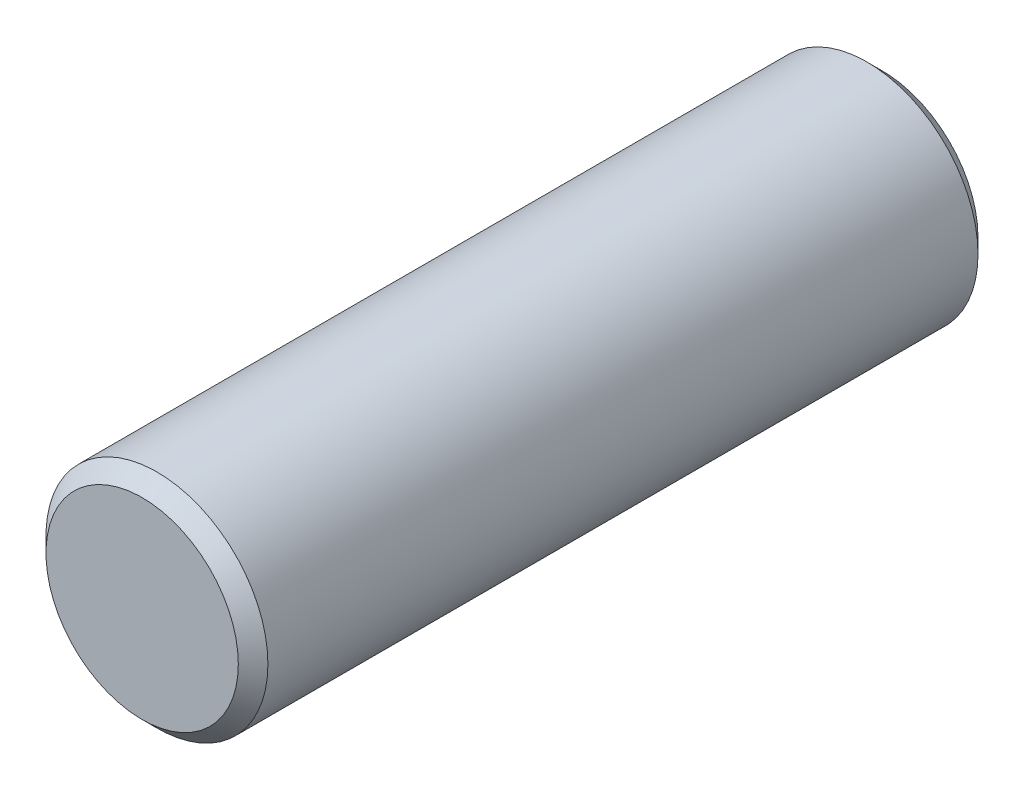
ISO-10303-21;
HEADER;
FILE_DESCRIPTION(('STEP AP214'),'2;1');
FILE_NAME('part.step','',(''),(''),'','','');
FILE_SCHEMA(('AUTOMOTIVE_DESIGN { 1 0 10303 214 1 1 1 1 }'));
ENDSEC;
DATA;
#1=APPLICATION_CONTEXT('core data for automotive mechanical design processes');
#2=APPLICATION_PROTOCOL_DEFINITION('international standard','automotive_design',2000,#1);
#3=PRODUCT_CONTEXT('',#1,'mechanical');
#4=PRODUCT('Part','Part','',(#3));
#5=PRODUCT_RELATED_PRODUCT_CATEGORY('part','',(#4));
#6=PRODUCT_DEFINITION_FORMATION('','',#4);
#7=PRODUCT_DEFINITION_CONTEXT('part definition',#1,'design');
#8=PRODUCT_DEFINITION('design','',#6,#7);
#9=PRODUCT_DEFINITION_SHAPE('','',#8);
#10=(LENGTH_UNIT() NAMED_UNIT(*) SI_UNIT(.MILLI.,.METRE.));
#11=(NAMED_UNIT(*) PLANE_ANGLE_UNIT() SI_UNIT($,.RADIAN.));
#12=(NAMED_UNIT(*) SI_UNIT($,.STERADIAN.) SOLID_ANGLE_UNIT());
#13=UNCERTAINTY_MEASURE_WITH_UNIT(LENGTH_MEASURE(1.E-05),#10,'distance_accuracy_value','');
#14=(GEOMETRIC_REPRESENTATION_CONTEXT(3) GLOBAL_UNCERTAINTY_ASSIGNED_CONTEXT((#13)) GLOBAL_UNIT_ASSIGNED_CONTEXT((#10,
#11,#12)) REPRESENTATION_CONTEXT('',''));
#15=CARTESIAN_POINT('',(0.,0.,0.));
#16=DIRECTION('',(0.,0.,1.));
#17=DIRECTION('',(1.,0.,0.));
#18=AXIS2_PLACEMENT_3D('',#15,#16,#17);
#19=CARTESIAN_POINT('',(0.,0.,5.));
#20=DIRECTION('',(0.,0.,-1.));
#21=DIRECTION('',(-1.,0.,0.));
#22=AXIS2_PLACEMENT_3D('',#19,#20,#21);
#23=CYLINDRICAL_SURFACE('',#22,1.5);
#24=CARTESIAN_POINT('',(0.,0.,-4.8));
#25=DIRECTION('',(0.,0.,1.));
#26=DIRECTION('',(1.,0.,0.));
#27=AXIS2_PLACEMENT_3D('',#24,#25,#26);
#28=CIRCLE('',#27,1.5);
#29=CARTESIAN_POINT('',(1.5,0.,-4.8));
#30=VERTEX_POINT('',#29);
#31=EDGE_CURVE('E51',#30,#30,#28,.T.);
#32=ORIENTED_EDGE('',*,*,#31,.T.);
#33=EDGE_LOOP('',(#32));
#34=FACE_BOUND('',#33,.T.);
#35=CARTESIAN_POINT('',(0.,0.,4.8));
#36=DIRECTION('',(0.,0.,1.));
#37=DIRECTION('',(1.,0.,0.));
#38=AXIS2_PLACEMENT_3D('',#35,#36,#37);
#39=CIRCLE('',#38,1.5);
#40=CARTESIAN_POINT('',(1.5,0.,4.8));
#41=VERTEX_POINT('',#40);
#42=EDGE_CURVE('E54',#41,#41,#39,.F.);
#43=ORIENTED_EDGE('',*,*,#42,.T.);
#44=EDGE_LOOP('',(#43));
#45=FACE_BOUND('',#44,.T.);
#46=ADVANCED_FACE('F39',(#34,#45),#23,.T.);
#47=CARTESIAN_POINT('',(0.,0.,5.));
#48=DIRECTION('',(0.,0.,1.));
#49=DIRECTION('',(1.,0.,0.));
#50=AXIS2_PLACEMENT_3D('',#47,#48,#49);
#51=PLANE('',#50);
#52=CARTESIAN_POINT('',(0.,0.,5.));
#53=DIRECTION('',(0.,0.,1.));
#54=DIRECTION('',(1.,0.,0.));
#55=AXIS2_PLACEMENT_3D('',#52,#53,#54);
#56=CIRCLE('',#55,1.3);
#57=CARTESIAN_POINT('',(1.3,0.,5.));
#58=VERTEX_POINT('',#57);
#59=EDGE_CURVE('E10',#58,#58,#56,.T.);
#60=ORIENTED_EDGE('',*,*,#59,.T.);
#61=EDGE_LOOP('',(#60));
#62=FACE_BOUND('',#61,.T.);
#63=ADVANCED_FACE('F72',(#62),#51,.T.);
#64=CARTESIAN_POINT('',(0.,0.,-5.));
#65=DIRECTION('',(0.,0.,1.));
#66=DIRECTION('',(1.,0.,0.));
#67=AXIS2_PLACEMENT_3D('',#64,#65,#66);
#68=PLANE('',#67);
#69=CARTESIAN_POINT('',(0.,0.,-5.));
#70=DIRECTION('',(0.,0.,1.));
#71=DIRECTION('',(1.,0.,0.));
#72=AXIS2_PLACEMENT_3D('',#69,#70,#71);
#73=CIRCLE('',#72,1.3);
#74=CARTESIAN_POINT('',(1.3,0.,-5.));
#75=VERTEX_POINT('',#74);
#76=EDGE_CURVE('E50',#75,#75,#73,.F.);
#77=ORIENTED_EDGE('',*,*,#76,.T.);
#78=EDGE_LOOP('',(#77));
#79=FACE_BOUND('',#78,.T.);
#80=ADVANCED_FACE('F70',(#79),#68,.F.);
#81=CARTESIAN_POINT('',(0.,0.,-4.8));
#82=DIRECTION('',(0.,0.,1.));
#83=DIRECTION('',(1.,0.,0.));
#84=AXIS2_PLACEMENT_3D('',#81,#82,#83);
#85=CONICAL_SURFACE('',#84,1.5,0.785398163397452);
#86=ORIENTED_EDGE('',*,*,#76,.F.);
#87=EDGE_LOOP('',(#86));
#88=FACE_BOUND('',#87,.T.);
#89=ORIENTED_EDGE('',*,*,#31,.F.);
#90=EDGE_LOOP('',(#89));
#91=FACE_BOUND('',#90,.T.);
#92=ADVANCED_FACE('F63',(#88,#91),#85,.T.);
#93=CARTESIAN_POINT('',(0.,0.,5.));
#94=DIRECTION('',(0.,0.,-1.));
#95=DIRECTION('',(-1.,0.,0.));
#96=AXIS2_PLACEMENT_3D('',#93,#94,#95);
#97=CONICAL_SURFACE('',#96,1.3,0.785398163397446);
#98=ORIENTED_EDGE('',*,*,#42,.F.);
#99=EDGE_LOOP('',(#98));
#100=FACE_BOUND('',#99,.T.);
#101=ORIENTED_EDGE('',*,*,#59,.F.);
#102=EDGE_LOOP('',(#101));
#103=FACE_BOUND('',#102,.T.);
#104=ADVANCED_FACE('F45',(#100,#103),#97,.T.);
#105=CLOSED_SHELL('',(#46,#63,#80,#92,#104));
#106=MANIFOLD_SOLID_BREP('B2',#105);
#107=ADVANCED_BREP_SHAPE_REPRESENTATION('',(#18,#106),#14);
#108=SHAPE_DEFINITION_REPRESENTATION(#9,#107);
ENDSEC;
END-ISO-10303-21;
